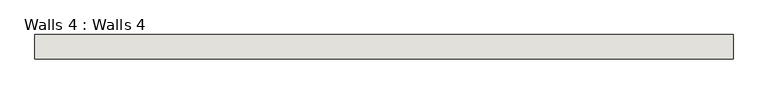
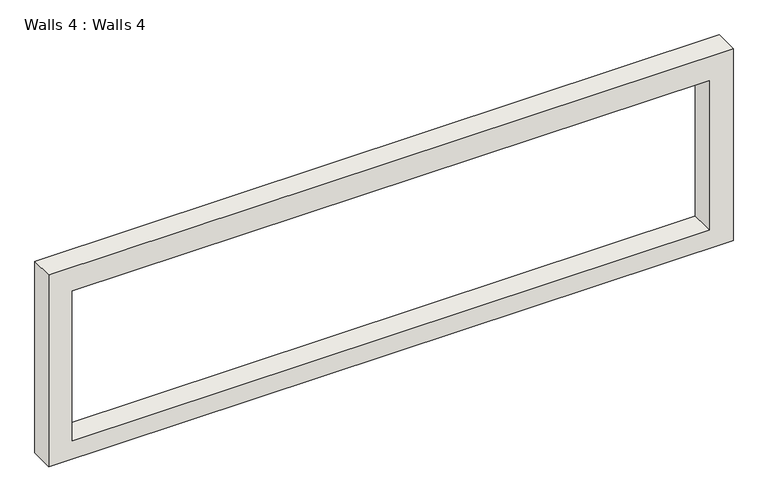
"""IFC4 building model written with IfcOpenShell, lengths in millimetres: wall geometry, Walls 4 : Walls 4."""

from ifc_helpers import new_model, si_unit, frame, origin, place, context, project, spatial, polyline, outline, extrude, source, transform, mapped, element, save


def walls_4_walls_4_69c7fff0(model_context):
    return source(origin(), model_context, "Body", "SweptSolid", [
        extrude(outline(polyline([(19431.0, -96.3561565), (19431.0, -8833.9561565), (16840.2, -8833.9561565), (16840.2, -96.3561565), (19431.0, -96.3561565)]), holes=[polyline([(19106.4577502, -401.1561565), (17087.4973119, -401.1561565), (17087.4973119, -8532.4946559), (19106.4577502, -8532.4946559), (19106.4577502, -401.1561565)])]), frame((0.0, 1191.8402851, 0.0), z_axis=(0.0, 1.0, 0.0), x_axis=(0.0, 0.0, 1.0)), (0.0, 0.0, 1.0), 304.8),
    ])


if __name__ == "__main__":
    model = new_model("IFC4")
    model_context = context("Model", 3, world=origin())
    ifc_project = project(units=[si_unit("LENGTHUNIT", "METRE", prefix="MILLI")], contexts=[model_context])
    site = spatial("IfcSite", under=ifc_project)
    building = spatial("IfcBuilding", under=site)
    placement = place(None, origin())
    walls_4_walls_4_shape = walls_4_walls_4_69c7fff0(model_context)
    element("IfcWall", 1, ObjectType="Walls 4 : Walls 4", at=placement, inside=building, context=model_context, shape_type="MappedRepresentation", body=[
        mapped(walls_4_walls_4_shape, transform((0.0, 0.0, 0.0), x_axis=(1.0, 0.0, 0.0), y_axis=(0.0, 1.0, 0.0), z_axis=(0.0, 0.0, 1.0))),
    ])
    save(model, "model.ifc")

# Revit data of these elements
# Element 1 (IfcWall, "Walls 4 : Walls 4")
#   Materials on its faces: "Default Wall"
# Materials
#   "Default Wall": colour RGB 128 128 128, transparency 0
